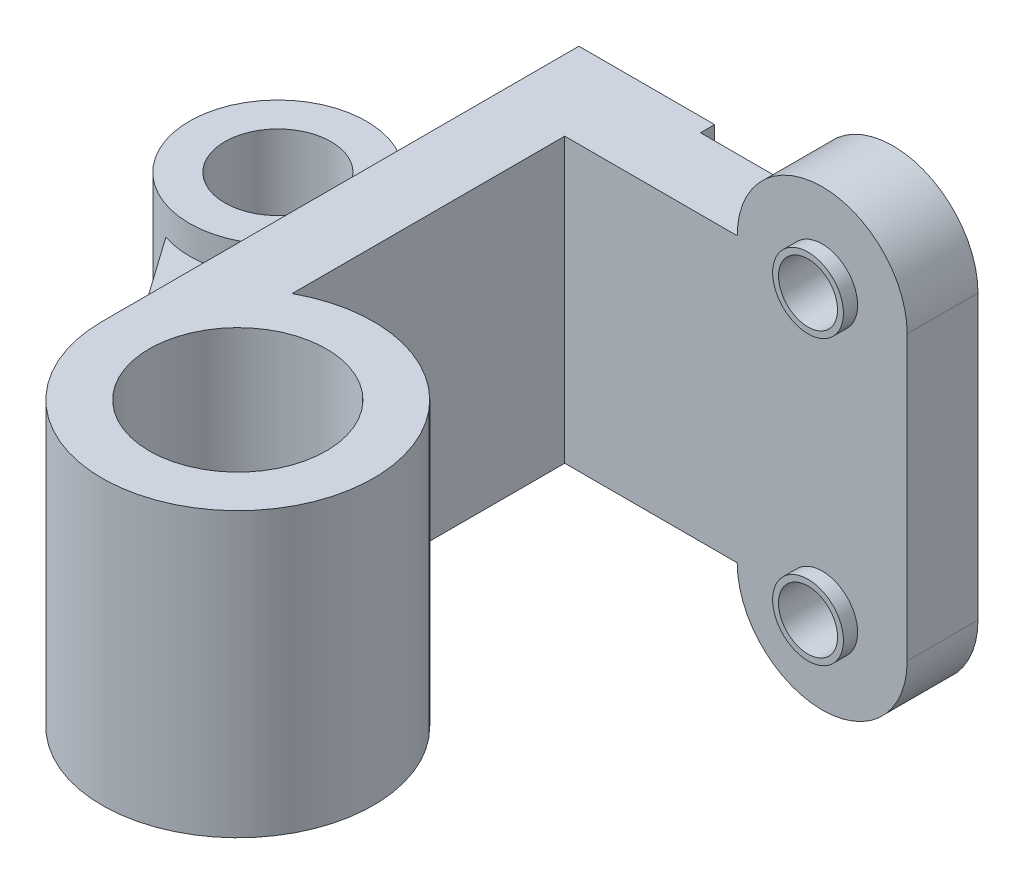
ISO-10303-21;
HEADER;
FILE_DESCRIPTION(('STEP AP214'),'2;1');
FILE_NAME('part.step','',(''),(''),'','','');
FILE_SCHEMA(('AUTOMOTIVE_DESIGN { 1 0 10303 214 1 1 1 1 }'));
ENDSEC;
DATA;
#1=APPLICATION_CONTEXT('core data for automotive mechanical design processes');
#2=APPLICATION_PROTOCOL_DEFINITION('international standard','automotive_design',2000,#1);
#3=PRODUCT_CONTEXT('',#1,'mechanical');
#4=PRODUCT('Part','Part','',(#3));
#5=PRODUCT_RELATED_PRODUCT_CATEGORY('part','',(#4));
#6=PRODUCT_DEFINITION_FORMATION('','',#4);
#7=PRODUCT_DEFINITION_CONTEXT('part definition',#1,'design');
#8=PRODUCT_DEFINITION('design','',#6,#7);
#9=PRODUCT_DEFINITION_SHAPE('','',#8);
#10=(LENGTH_UNIT() NAMED_UNIT(*) SI_UNIT(.MILLI.,.METRE.));
#11=(NAMED_UNIT(*) PLANE_ANGLE_UNIT() SI_UNIT($,.RADIAN.));
#12=(NAMED_UNIT(*) SI_UNIT($,.STERADIAN.) SOLID_ANGLE_UNIT());
#13=UNCERTAINTY_MEASURE_WITH_UNIT(LENGTH_MEASURE(1.E-05),#10,'distance_accuracy_value','');
#14=(GEOMETRIC_REPRESENTATION_CONTEXT(3) GLOBAL_UNCERTAINTY_ASSIGNED_CONTEXT((#13)) GLOBAL_UNIT_ASSIGNED_CONTEXT((#10,
#11,#12)) REPRESENTATION_CONTEXT('',''));
#15=CARTESIAN_POINT('',(0.,0.,0.));
#16=DIRECTION('',(0.,0.,1.));
#17=DIRECTION('',(1.,0.,0.));
#18=AXIS2_PLACEMENT_3D('',#15,#16,#17);
#19=CARTESIAN_POINT('',(-25.3130662470469,13.,-35.3301610889812));
#20=DIRECTION('',(0.582414315015222,0.,0.812892099645058));
#21=DIRECTION('',(0.812892099645058,0.,-0.582414315015222));
#22=AXIS2_PLACEMENT_3D('',#19,#20,#21);
#23=PLANE('',#22);
#24=DIRECTION('',(0.,-1.,0.));
#25=VECTOR('',#24,1.);
#26=CARTESIAN_POINT('',(-118.590283261648,25.,31.5003401273626));
#27=LINE('',#26,#25);
#28=CARTESIAN_POINT('',(-118.590283261648,13.,31.5003401273626));
#29=VERTEX_POINT('',#28);
#30=CARTESIAN_POINT('',(-118.590283261648,-13.,31.5003401273626));
#31=VERTEX_POINT('',#30);
#32=EDGE_CURVE('E61',#29,#31,#27,.T.);
#33=ORIENTED_EDGE('',*,*,#32,.F.);
#34=DIRECTION('',(-0.812892099645058,0.,0.582414315015222));
#35=VECTOR('',#34,1.);
#36=CARTESIAN_POINT('',(-25.3130662470469,13.,-35.3301610889812));
#37=LINE('',#36,#35);
#38=CARTESIAN_POINT('',(-66.25,13.,-6.));
#39=VERTEX_POINT('',#38);
#40=EDGE_CURVE('E170',#39,#29,#37,.T.);
#41=ORIENTED_EDGE('',*,*,#40,.F.);
#42=DIRECTION('',(0.,-1.,0.));
#43=VECTOR('',#42,1.);
#44=CARTESIAN_POINT('',(-66.25,13.,-6.));
#45=LINE('',#44,#43);
#46=CARTESIAN_POINT('',(-66.25,-13.,-6.));
#47=VERTEX_POINT('',#46);
#48=EDGE_CURVE('E175',#39,#47,#45,.T.);
#49=ORIENTED_EDGE('',*,*,#48,.T.);
#50=DIRECTION('',(-0.812892099645058,0.,0.582414315015222));
#51=VECTOR('',#50,1.);
#52=CARTESIAN_POINT('',(-25.3130662470469,-13.,-35.3301610889812));
#53=LINE('',#52,#51);
#54=EDGE_CURVE('E155',#47,#31,#53,.T.);
#55=ORIENTED_EDGE('',*,*,#54,.T.);
#56=EDGE_LOOP('',(#33,#41,#49,#55));
#57=FACE_BOUND('',#56,.T.);
#58=ADVANCED_FACE('F41',(#57),#23,.F.);
#59=CARTESIAN_POINT('',(-136.555750036393,13.,96.170909540454));
#60=DIRECTION('',(-0.81759186098535,0.,0.575798184132697));
#61=DIRECTION('',(0.575798184132697,0.,0.81759186098535));
#62=AXIS2_PLACEMENT_3D('',#59,#60,#61);
#63=PLANE('',#62);
#64=DIRECTION('',(-0.575798184132697,0.,-0.81759186098535));
#65=VECTOR('',#64,1.);
#66=CARTESIAN_POINT('',(-136.555750036393,13.,96.170909540454));
#67=LINE('',#66,#65);
#68=CARTESIAN_POINT('',(-66.25,13.,196.));
#69=VERTEX_POINT('',#68);
#70=CARTESIAN_POINT('',(-130.645274515728,13.,104.563358168141));
#71=VERTEX_POINT('',#70);
#72=EDGE_CURVE('E160',#69,#71,#67,.T.);
#73=ORIENTED_EDGE('',*,*,#72,.T.);
#74=DIRECTION('',(0.,-1.,0.));
#75=VECTOR('',#74,1.);
#76=CARTESIAN_POINT('',(-130.645274515728,25.,104.563358168141));
#77=LINE('',#76,#75);
#78=CARTESIAN_POINT('',(-130.645274515728,-13.,104.563358168141));
#79=VERTEX_POINT('',#78);
#80=EDGE_CURVE('E152',#71,#79,#77,.T.);
#81=ORIENTED_EDGE('',*,*,#80,.T.);
#82=DIRECTION('',(-0.575798184132697,0.,-0.81759186098535));
#83=VECTOR('',#82,1.);
#84=CARTESIAN_POINT('',(-136.555750036393,-13.,96.170909540454));
#85=LINE('',#84,#83);
#86=CARTESIAN_POINT('',(-66.25,-13.,196.));
#87=VERTEX_POINT('',#86);
#88=EDGE_CURVE('E144',#87,#79,#85,.T.);
#89=ORIENTED_EDGE('',*,*,#88,.F.);
#90=DIRECTION('',(0.,-1.,0.));
#91=VECTOR('',#90,1.);
#92=CARTESIAN_POINT('',(-66.25,13.,196.));
#93=LINE('',#92,#91);
#94=EDGE_CURVE('E176',#69,#87,#93,.T.);
#95=ORIENTED_EDGE('',*,*,#94,.F.);
#96=EDGE_LOOP('',(#73,#81,#89,#95));
#97=FACE_BOUND('',#96,.T.);
#98=ADVANCED_FACE('F158',(#97),#63,.T.);
#99=CARTESIAN_POINT('',(-66.25,60.,30.));
#100=DIRECTION('',(1.,0.,0.));
#101=DIRECTION('',(0.,0.,-1.));
#102=AXIS2_PLACEMENT_3D('',#99,#100,#101);
#103=PLANE('',#102);
#104=DIRECTION('',(0.,0.,-1.));
#105=VECTOR('',#104,1.);
#106=CARTESIAN_POINT('',(-66.25,-13.,0.));
#107=LINE('',#106,#105);
#108=EDGE_CURVE('E146',#87,#47,#107,.T.);
#109=ORIENTED_EDGE('',*,*,#108,.T.);
#110=DIRECTION('',(0.,-1.,0.));
#111=VECTOR('',#110,1.);
#112=CARTESIAN_POINT('',(-66.25,60.,-6.));
#113=LINE('',#112,#111);
#114=CARTESIAN_POINT('',(-66.25,-60.,-6.));
#115=VERTEX_POINT('',#114);
#116=EDGE_CURVE('E214',#47,#115,#113,.T.);
#117=ORIENTED_EDGE('',*,*,#116,.T.);
#118=DIRECTION('',(0.,0.,-1.));
#119=VECTOR('',#118,1.);
#120=CARTESIAN_POINT('',(-66.25,-60.,30.));
#121=LINE('',#120,#119);
#122=CARTESIAN_POINT('',(-66.25,-60.,196.));
#123=VERTEX_POINT('',#122);
#124=EDGE_CURVE('E285',#123,#115,#121,.T.);
#125=ORIENTED_EDGE('',*,*,#124,.F.);
#126=DIRECTION('',(0.,-1.,0.));
#127=VECTOR('',#126,1.);
#128=CARTESIAN_POINT('',(-66.25,0.,196.));
#129=LINE('',#128,#127);
#130=EDGE_CURVE('E199',#87,#123,#129,.T.);
#131=ORIENTED_EDGE('',*,*,#130,.F.);
#132=EDGE_LOOP('',(#109,#117,#125,#131));
#133=FACE_BOUND('',#132,.T.);
#134=ADVANCED_FACE('F357',(#133),#103,.F.);
#135=CARTESIAN_POINT('',(-36.25,0.,196.));
#136=DIRECTION('',(1.,0.,0.));
#137=DIRECTION('',(0.,1.,0.));
#138=AXIS2_PLACEMENT_3D('',#135,#136,#137);
#139=PLANE('',#138);
#140=DIRECTION('',(0.,0.,-1.));
#141=VECTOR('',#140,1.);
#142=CARTESIAN_POINT('',(-36.25,60.,196.));
#143=LINE('',#142,#141);
#144=CARTESIAN_POINT('',(-36.25,60.,145.50247530819));
#145=VERTEX_POINT('',#144);
#146=CARTESIAN_POINT('',(-36.25,60.,30.));
#147=VERTEX_POINT('',#146);
#148=EDGE_CURVE('E201',#145,#147,#143,.T.);
#149=ORIENTED_EDGE('',*,*,#148,.F.);
#150=DIRECTION('',(0.,-1.,0.));
#151=VECTOR('',#150,1.);
#152=CARTESIAN_POINT('',(-36.25,60.,145.50247530819));
#153=LINE('',#152,#151);
#154=CARTESIAN_POINT('',(-36.25,-60.,145.50247530819));
#155=VERTEX_POINT('',#154);
#156=EDGE_CURVE('E190',#145,#155,#153,.T.);
#157=ORIENTED_EDGE('',*,*,#156,.T.);
#158=DIRECTION('',(0.,0.,-1.));
#159=VECTOR('',#158,1.);
#160=CARTESIAN_POINT('',(-36.25,-60.,196.));
#161=LINE('',#160,#159);
#162=CARTESIAN_POINT('',(-36.25,-60.,30.));
#163=VERTEX_POINT('',#162);
#164=EDGE_CURVE('E196',#155,#163,#161,.T.);
#165=ORIENTED_EDGE('',*,*,#164,.T.);
#166=DIRECTION('',(0.,-1.,0.));
#167=VECTOR('',#166,1.);
#168=CARTESIAN_POINT('',(-36.25,0.,30.));
#169=LINE('',#168,#167);
#170=EDGE_CURVE('E191',#147,#163,#169,.T.);
#171=ORIENTED_EDGE('',*,*,#170,.F.);
#172=EDGE_LOOP('',(#149,#157,#165,#171));
#173=FACE_BOUND('',#172,.T.);
#174=ADVANCED_FACE('F321',(#173),#139,.T.);
#175=CARTESIAN_POINT('',(72.8125,60.,0.));
#176=DIRECTION('',(0.,0.,1.));
#177=DIRECTION('',(1.,0.,0.));
#178=AXIS2_PLACEMENT_3D('',#175,#176,#177);
#179=PLANE('',#178);
#180=CARTESIAN_POINT('',(72.8125,-60.,0.));
#181=DIRECTION('',(0.,0.,1.));
#182=DIRECTION('',(1.,0.,0.));
#183=AXIS2_PLACEMENT_3D('',#180,#181,#182);
#184=CIRCLE('',#183,12.5);
#185=CARTESIAN_POINT('',(85.3125,-60.,0.));
#186=VERTEX_POINT('',#185);
#187=EDGE_CURVE('E241',#186,#186,#184,.T.);
#188=ORIENTED_EDGE('',*,*,#187,.T.);
#189=EDGE_LOOP('',(#188));
#190=FACE_BOUND('',#189,.T.);
#191=CARTESIAN_POINT('',(72.8125,60.,0.));
#192=DIRECTION('',(0.,0.,1.));
#193=DIRECTION('',(1.,0.,0.));
#194=AXIS2_PLACEMENT_3D('',#191,#192,#193);
#195=CIRCLE('',#194,12.5);
#196=CARTESIAN_POINT('',(85.3125,60.,0.));
#197=VERTEX_POINT('',#196);
#198=EDGE_CURVE('E246',#197,#197,#195,.T.);
#199=ORIENTED_EDGE('',*,*,#198,.T.);
#200=EDGE_LOOP('',(#199));
#201=FACE_BOUND('',#200,.T.);
#202=DIRECTION('',(0.,-1.,0.));
#203=VECTOR('',#202,1.);
#204=CARTESIAN_POINT('',(-8.75,60.,0.));
#205=LINE('',#204,#203);
#206=CARTESIAN_POINT('',(-8.75000000000001,60.,0.));
#207=VERTEX_POINT('',#206);
#208=CARTESIAN_POINT('',(-8.75000000000001,-60.,0.));
#209=VERTEX_POINT('',#208);
#210=EDGE_CURVE('E202',#207,#209,#205,.T.);
#211=ORIENTED_EDGE('',*,*,#210,.F.);
#212=DIRECTION('',(-1.,0.,0.));
#213=VECTOR('',#212,1.);
#214=CARTESIAN_POINT('',(36.8125,60.,0.));
#215=LINE('',#214,#213);
#216=CARTESIAN_POINT('',(36.8125,60.,0.));
#217=VERTEX_POINT('',#216);
#218=EDGE_CURVE('E268',#217,#207,#215,.T.);
#219=ORIENTED_EDGE('',*,*,#218,.F.);
#220=CARTESIAN_POINT('',(72.8125,60.,0.));
#221=DIRECTION('',(0.,0.,1.));
#222=DIRECTION('',(1.,0.,0.));
#223=AXIS2_PLACEMENT_3D('',#220,#221,#222);
#224=CIRCLE('',#223,36.);
#225=CARTESIAN_POINT('',(108.8125,60.,0.));
#226=VERTEX_POINT('',#225);
#227=EDGE_CURVE('E248',#226,#217,#224,.T.);
#228=ORIENTED_EDGE('',*,*,#227,.F.);
#229=DIRECTION('',(0.,1.,0.));
#230=VECTOR('',#229,1.);
#231=CARTESIAN_POINT('',(108.8125,60.,0.));
#232=LINE('',#231,#230);
#233=CARTESIAN_POINT('',(108.8125,-60.,0.));
#234=VERTEX_POINT('',#233);
#235=EDGE_CURVE('E251',#234,#226,#232,.T.);
#236=ORIENTED_EDGE('',*,*,#235,.F.);
#237=CARTESIAN_POINT('',(72.8125,-60.,0.));
#238=DIRECTION('',(0.,0.,1.));
#239=DIRECTION('',(1.,0.,0.));
#240=AXIS2_PLACEMENT_3D('',#237,#238,#239);
#241=CIRCLE('',#240,36.);
#242=CARTESIAN_POINT('',(36.8125,-60.,0.));
#243=VERTEX_POINT('',#242);
#244=EDGE_CURVE('E272',#243,#234,#241,.T.);
#245=ORIENTED_EDGE('',*,*,#244,.F.);
#246=DIRECTION('',(1.,0.,0.));
#247=VECTOR('',#246,1.);
#248=CARTESIAN_POINT('',(-66.25,-60.,0.));
#249=LINE('',#248,#247);
#250=EDGE_CURVE('E269',#209,#243,#249,.T.);
#251=ORIENTED_EDGE('',*,*,#250,.F.);
#252=EDGE_LOOP('',(#211,#219,#228,#236,#245,#251));
#253=FACE_BOUND('',#252,.T.);
#254=ADVANCED_FACE('F296',(#190,#201,#253),#179,.F.);
#255=CARTESIAN_POINT('',(72.8125,60.,30.));
#256=DIRECTION('',(0.,0.,1.));
#257=DIRECTION('',(1.,0.,0.));
#258=AXIS2_PLACEMENT_3D('',#255,#256,#257);
#259=PLANE('',#258);
#260=ORIENTED_EDGE('',*,*,#170,.T.);
#261=DIRECTION('',(1.,0.,0.));
#262=VECTOR('',#261,1.);
#263=CARTESIAN_POINT('',(-66.25,-60.,30.));
#264=LINE('',#263,#262);
#265=CARTESIAN_POINT('',(36.8125,-60.,30.));
#266=VERTEX_POINT('',#265);
#267=EDGE_CURVE('E260',#163,#266,#264,.T.);
#268=ORIENTED_EDGE('',*,*,#267,.T.);
#269=CARTESIAN_POINT('',(72.8125,-60.,30.));
#270=DIRECTION('',(0.,0.,1.));
#271=DIRECTION('',(1.,0.,0.));
#272=AXIS2_PLACEMENT_3D('',#269,#270,#271);
#273=CIRCLE('',#272,36.);
#274=CARTESIAN_POINT('',(108.8125,-60.,30.));
#275=VERTEX_POINT('',#274);
#276=EDGE_CURVE('E256',#266,#275,#273,.T.);
#277=ORIENTED_EDGE('',*,*,#276,.T.);
#278=DIRECTION('',(0.,1.,0.));
#279=VECTOR('',#278,1.);
#280=CARTESIAN_POINT('',(108.8125,60.,30.));
#281=LINE('',#280,#279);
#282=CARTESIAN_POINT('',(108.8125,60.,30.));
#283=VERTEX_POINT('',#282);
#284=EDGE_CURVE('E263',#275,#283,#281,.T.);
#285=ORIENTED_EDGE('',*,*,#284,.T.);
#286=CARTESIAN_POINT('',(72.8125,60.,30.));
#287=DIRECTION('',(0.,0.,1.));
#288=DIRECTION('',(1.,0.,0.));
#289=AXIS2_PLACEMENT_3D('',#286,#287,#288);
#290=CIRCLE('',#289,36.);
#291=CARTESIAN_POINT('',(36.8125,60.,30.));
#292=VERTEX_POINT('',#291);
#293=EDGE_CURVE('E249',#283,#292,#290,.T.);
#294=ORIENTED_EDGE('',*,*,#293,.T.);
#295=DIRECTION('',(-1.,0.,0.));
#296=VECTOR('',#295,1.);
#297=CARTESIAN_POINT('',(36.8125,60.,30.));
#298=LINE('',#297,#296);
#299=EDGE_CURVE('E254',#292,#147,#298,.T.);
#300=ORIENTED_EDGE('',*,*,#299,.T.);
#301=EDGE_LOOP('',(#260,#268,#277,#285,#294,#300));
#302=FACE_BOUND('',#301,.T.);
#303=CARTESIAN_POINT('',(72.8125,-60.,30.));
#304=DIRECTION('',(0.,0.,1.));
#305=DIRECTION('',(1.,0.,0.));
#306=AXIS2_PLACEMENT_3D('',#303,#304,#305);
#307=CIRCLE('',#306,15.);
#308=CARTESIAN_POINT('',(87.8125,-60.,30.));
#309=VERTEX_POINT('',#308);
#310=EDGE_CURVE('E230',#309,#309,#307,.T.);
#311=ORIENTED_EDGE('',*,*,#310,.F.);
#312=EDGE_LOOP('',(#311));
#313=FACE_BOUND('',#312,.T.);
#314=CARTESIAN_POINT('',(72.8125,60.,30.));
#315=DIRECTION('',(0.,0.,1.));
#316=DIRECTION('',(1.,0.,0.));
#317=AXIS2_PLACEMENT_3D('',#314,#315,#316);
#318=CIRCLE('',#317,15.);
#319=CARTESIAN_POINT('',(87.8125,60.,30.));
#320=VERTEX_POINT('',#319);
#321=EDGE_CURVE('E232',#320,#320,#318,.T.);
#322=ORIENTED_EDGE('',*,*,#321,.F.);
#323=EDGE_LOOP('',(#322));
#324=FACE_BOUND('',#323,.T.);
#325=ADVANCED_FACE('F325',(#302,#313,#324),#259,.T.);
#326=CARTESIAN_POINT('',(72.8125,60.,30.));
#327=DIRECTION('',(0.,0.,-1.));
#328=DIRECTION('',(-1.,0.,0.));
#329=AXIS2_PLACEMENT_3D('',#326,#327,#328);
#330=CYLINDRICAL_SURFACE('',#329,36.);
#331=ORIENTED_EDGE('',*,*,#227,.T.);
#332=DIRECTION('',(0.,0.,-1.));
#333=VECTOR('',#332,1.);
#334=CARTESIAN_POINT('',(36.8125,60.,30.));
#335=LINE('',#334,#333);
#336=EDGE_CURVE('E47',#292,#217,#335,.T.);
#337=ORIENTED_EDGE('',*,*,#336,.F.);
#338=ORIENTED_EDGE('',*,*,#293,.F.);
#339=DIRECTION('',(0.,0.,-1.));
#340=VECTOR('',#339,1.);
#341=CARTESIAN_POINT('',(108.8125,60.,30.));
#342=LINE('',#341,#340);
#343=EDGE_CURVE('E261',#283,#226,#342,.T.);
#344=ORIENTED_EDGE('',*,*,#343,.T.);
#345=EDGE_LOOP('',(#331,#337,#338,#344));
#346=FACE_BOUND('',#345,.T.);
#347=ADVANCED_FACE('F43',(#346),#330,.T.);
#348=CARTESIAN_POINT('',(36.8125,60.,30.));
#349=DIRECTION('',(0.,-1.,0.));
#350=DIRECTION('',(0.,0.,-1.));
#351=AXIS2_PLACEMENT_3D('',#348,#349,#350);
#352=PLANE('',#351);
#353=DIRECTION('',(0.,0.,-1.));
#354=VECTOR('',#353,1.);
#355=CARTESIAN_POINT('',(-66.25,60.,30.));
#356=LINE('',#355,#354);
#357=CARTESIAN_POINT('',(-66.25,60.,196.));
#358=VERTEX_POINT('',#357);
#359=CARTESIAN_POINT('',(-66.25,60.,-6.));
#360=VERTEX_POINT('',#359);
#361=EDGE_CURVE('E282',#358,#360,#356,.T.);
#362=ORIENTED_EDGE('',*,*,#361,.F.);
#363=CARTESIAN_POINT('',(-8.75,60.,196.));
#364=DIRECTION('',(0.,1.,0.));
#365=DIRECTION('',(0.,0.,1.));
#366=AXIS2_PLACEMENT_3D('',#363,#364,#365);
#367=CIRCLE('',#366,57.5);
#368=EDGE_CURVE('E182',#358,#145,#367,.T.);
#369=ORIENTED_EDGE('',*,*,#368,.T.);
#370=ORIENTED_EDGE('',*,*,#148,.T.);
#371=ORIENTED_EDGE('',*,*,#299,.F.);
#372=ORIENTED_EDGE('',*,*,#336,.T.);
#373=ORIENTED_EDGE('',*,*,#218,.T.);
#374=DIRECTION('',(0.,0.,1.));
#375=VECTOR('',#374,1.);
#376=CARTESIAN_POINT('',(-8.75,60.,-6.));
#377=LINE('',#376,#375);
#378=CARTESIAN_POINT('',(-8.75,60.,-6.));
#379=VERTEX_POINT('',#378);
#380=EDGE_CURVE('E217',#379,#207,#377,.T.);
#381=ORIENTED_EDGE('',*,*,#380,.F.);
#382=DIRECTION('',(1.,0.,0.));
#383=VECTOR('',#382,1.);
#384=CARTESIAN_POINT('',(-66.25,60.,-6.));
#385=LINE('',#384,#383);
#386=EDGE_CURVE('E212',#360,#379,#385,.T.);
#387=ORIENTED_EDGE('',*,*,#386,.F.);
#388=EDGE_LOOP('',(#362,#369,#370,#371,#372,#373,#381,#387));
#389=FACE_BOUND('',#388,.T.);
#390=CARTESIAN_POINT('',(-8.75,60.,196.));
#391=DIRECTION('',(0.,1.,0.));
#392=DIRECTION('',(0.,0.,1.));
#393=AXIS2_PLACEMENT_3D('',#390,#391,#392);
#394=CIRCLE('',#393,37.5);
#395=CARTESIAN_POINT('',(-8.75,60.,233.5));
#396=VERTEX_POINT('',#395);
#397=EDGE_CURVE('E179',#396,#396,#394,.T.);
#398=ORIENTED_EDGE('',*,*,#397,.F.);
#399=EDGE_LOOP('',(#398));
#400=FACE_BOUND('',#399,.T.);
#401=ADVANCED_FACE('F289',(#389,#400),#352,.F.);
#402=EDGE_CURVE('E211',#360,#39,#113,.T.);
#403=ORIENTED_EDGE('',*,*,#402,.T.);
#404=DIRECTION('',(0.,0.,-1.));
#405=VECTOR('',#404,1.);
#406=CARTESIAN_POINT('',(-66.25,13.,0.));
#407=LINE('',#406,#405);
#408=EDGE_CURVE('E167',#69,#39,#407,.T.);
#409=ORIENTED_EDGE('',*,*,#408,.F.);
#410=EDGE_CURVE('E193',#358,#69,#129,.T.);
#411=ORIENTED_EDGE('',*,*,#410,.F.);
#412=ORIENTED_EDGE('',*,*,#361,.T.);
#413=EDGE_LOOP('',(#403,#409,#411,#412));
#414=FACE_BOUND('',#413,.T.);
#415=ADVANCED_FACE('F313',(#414),#103,.F.);
#416=CARTESIAN_POINT('',(-66.25,-60.,30.));
#417=DIRECTION('',(0.,1.,0.));
#418=DIRECTION('',(0.,0.,1.));
#419=AXIS2_PLACEMENT_3D('',#416,#417,#418);
#420=PLANE('',#419);
#421=ORIENTED_EDGE('',*,*,#164,.F.);
#422=CARTESIAN_POINT('',(-8.75,-60.,196.));
#423=DIRECTION('',(0.,1.,0.));
#424=DIRECTION('',(0.,0.,1.));
#425=AXIS2_PLACEMENT_3D('',#422,#423,#424);
#426=CIRCLE('',#425,57.5);
#427=EDGE_CURVE('E183',#123,#155,#426,.T.);
#428=ORIENTED_EDGE('',*,*,#427,.F.);
#429=ORIENTED_EDGE('',*,*,#124,.T.);
#430=DIRECTION('',(1.,0.,0.));
#431=VECTOR('',#430,1.);
#432=CARTESIAN_POINT('',(-66.25,-60.,-6.));
#433=LINE('',#432,#431);
#434=CARTESIAN_POINT('',(-8.75000000000001,-60.,-6.));
#435=VERTEX_POINT('',#434);
#436=EDGE_CURVE('E207',#115,#435,#433,.T.);
#437=ORIENTED_EDGE('',*,*,#436,.T.);
#438=DIRECTION('',(0.,0.,1.));
#439=VECTOR('',#438,1.);
#440=CARTESIAN_POINT('',(-8.75000000000001,-60.,-6.));
#441=LINE('',#440,#439);
#442=EDGE_CURVE('E220',#435,#209,#441,.T.);
#443=ORIENTED_EDGE('',*,*,#442,.T.);
#444=ORIENTED_EDGE('',*,*,#250,.T.);
#445=DIRECTION('',(0.,0.,-1.));
#446=VECTOR('',#445,1.);
#447=CARTESIAN_POINT('',(36.8125,-60.,30.));
#448=LINE('',#447,#446);
#449=EDGE_CURVE('E276',#266,#243,#448,.T.);
#450=ORIENTED_EDGE('',*,*,#449,.F.);
#451=ORIENTED_EDGE('',*,*,#267,.F.);
#452=EDGE_LOOP('',(#421,#428,#429,#437,#443,#444,#450,#451));
#453=FACE_BOUND('',#452,.T.);
#454=CARTESIAN_POINT('',(-8.75,-60.,196.));
#455=DIRECTION('',(0.,1.,0.));
#456=DIRECTION('',(0.,0.,1.));
#457=AXIS2_PLACEMENT_3D('',#454,#455,#456);
#458=CIRCLE('',#457,37.5);
#459=CARTESIAN_POINT('',(-8.75,-60.,233.5));
#460=VERTEX_POINT('',#459);
#461=EDGE_CURVE('E177',#460,#460,#458,.T.);
#462=ORIENTED_EDGE('',*,*,#461,.T.);
#463=EDGE_LOOP('',(#462));
#464=FACE_BOUND('',#463,.T.);
#465=ADVANCED_FACE('F329',(#453,#464),#420,.F.);
#466=CARTESIAN_POINT('',(72.8125,-60.,30.));
#467=DIRECTION('',(0.,0.,-1.));
#468=DIRECTION('',(-1.,0.,0.));
#469=AXIS2_PLACEMENT_3D('',#466,#467,#468);
#470=CYLINDRICAL_SURFACE('',#469,36.);
#471=ORIENTED_EDGE('',*,*,#244,.T.);
#472=DIRECTION('',(0.,0.,-1.));
#473=VECTOR('',#472,1.);
#474=CARTESIAN_POINT('',(108.8125,-60.,30.));
#475=LINE('',#474,#473);
#476=EDGE_CURVE('E277',#275,#234,#475,.T.);
#477=ORIENTED_EDGE('',*,*,#476,.F.);
#478=ORIENTED_EDGE('',*,*,#276,.F.);
#479=ORIENTED_EDGE('',*,*,#449,.T.);
#480=EDGE_LOOP('',(#471,#477,#478,#479));
#481=FACE_BOUND('',#480,.T.);
#482=ADVANCED_FACE('F332',(#481),#470,.T.);
#483=CARTESIAN_POINT('',(108.8125,60.,30.));
#484=DIRECTION('',(-1.,0.,0.));
#485=DIRECTION('',(0.,0.,1.));
#486=AXIS2_PLACEMENT_3D('',#483,#484,#485);
#487=PLANE('',#486);
#488=ORIENTED_EDGE('',*,*,#235,.T.);
#489=ORIENTED_EDGE('',*,*,#343,.F.);
#490=ORIENTED_EDGE('',*,*,#284,.F.);
#491=ORIENTED_EDGE('',*,*,#476,.T.);
#492=EDGE_LOOP('',(#488,#489,#490,#491));
#493=FACE_BOUND('',#492,.T.);
#494=ADVANCED_FACE('F340',(#493),#487,.F.);
#495=CARTESIAN_POINT('',(72.8125,60.,30.));
#496=DIRECTION('',(0.,0.,-1.));
#497=DIRECTION('',(-1.,0.,0.));
#498=AXIS2_PLACEMENT_3D('',#495,#496,#497);
#499=CYLINDRICAL_SURFACE('',#498,12.5);
#500=ORIENTED_EDGE('',*,*,#198,.F.);
#501=EDGE_LOOP('',(#500));
#502=FACE_BOUND('',#501,.T.);
#503=CARTESIAN_POINT('',(72.8125,60.,36.));
#504=DIRECTION('',(0.,0.,-1.));
#505=DIRECTION('',(-1.,0.,0.));
#506=AXIS2_PLACEMENT_3D('',#503,#504,#505);
#507=CIRCLE('',#506,12.5);
#508=CARTESIAN_POINT('',(60.3125,60.,36.));
#509=VERTEX_POINT('',#508);
#510=EDGE_CURVE('E228',#509,#509,#507,.T.);
#511=ORIENTED_EDGE('',*,*,#510,.F.);
#512=EDGE_LOOP('',(#511));
#513=FACE_BOUND('',#512,.T.);
#514=ADVANCED_FACE('F339',(#502,#513),#499,.F.);
#515=CARTESIAN_POINT('',(72.8125,-60.,30.));
#516=DIRECTION('',(0.,0.,-1.));
#517=DIRECTION('',(-1.,0.,0.));
#518=AXIS2_PLACEMENT_3D('',#515,#516,#517);
#519=CYLINDRICAL_SURFACE('',#518,12.5);
#520=ORIENTED_EDGE('',*,*,#187,.F.);
#521=EDGE_LOOP('',(#520));
#522=FACE_BOUND('',#521,.T.);
#523=CARTESIAN_POINT('',(72.8125,-60.,36.));
#524=DIRECTION('',(0.,0.,-1.));
#525=DIRECTION('',(-1.,0.,0.));
#526=AXIS2_PLACEMENT_3D('',#523,#524,#525);
#527=CIRCLE('',#526,12.5);
#528=CARTESIAN_POINT('',(60.3125,-60.,36.));
#529=VERTEX_POINT('',#528);
#530=EDGE_CURVE('E221',#529,#529,#527,.T.);
#531=ORIENTED_EDGE('',*,*,#530,.F.);
#532=EDGE_LOOP('',(#531));
#533=FACE_BOUND('',#532,.T.);
#534=ADVANCED_FACE('F348',(#522,#533),#519,.F.);
#535=CARTESIAN_POINT('',(72.8125,60.,36.));
#536=DIRECTION('',(0.,0.,-1.));
#537=DIRECTION('',(-1.,0.,0.));
#538=AXIS2_PLACEMENT_3D('',#535,#536,#537);
#539=CYLINDRICAL_SURFACE('',#538,15.);
#540=CARTESIAN_POINT('',(72.8125,60.,36.));
#541=DIRECTION('',(0.,0.,1.));
#542=DIRECTION('',(1.,0.,0.));
#543=AXIS2_PLACEMENT_3D('',#540,#541,#542);
#544=CIRCLE('',#543,15.);
#545=CARTESIAN_POINT('',(87.8125,60.,36.));
#546=VERTEX_POINT('',#545);
#547=EDGE_CURVE('E238',#546,#546,#544,.T.);
#548=ORIENTED_EDGE('',*,*,#547,.F.);
#549=EDGE_LOOP('',(#548));
#550=FACE_BOUND('',#549,.T.);
#551=ORIENTED_EDGE('',*,*,#321,.T.);
#552=EDGE_LOOP('',(#551));
#553=FACE_BOUND('',#552,.T.);
#554=ADVANCED_FACE('F381',(#550,#553),#539,.T.);
#555=CARTESIAN_POINT('',(72.8125,60.,36.));
#556=DIRECTION('',(0.,0.,1.));
#557=DIRECTION('',(1.,0.,0.));
#558=AXIS2_PLACEMENT_3D('',#555,#556,#557);
#559=PLANE('',#558);
#560=ORIENTED_EDGE('',*,*,#510,.T.);
#561=EDGE_LOOP('',(#560));
#562=FACE_BOUND('',#561,.T.);
#563=ORIENTED_EDGE('',*,*,#547,.T.);
#564=EDGE_LOOP('',(#563));
#565=FACE_BOUND('',#564,.T.);
#566=ADVANCED_FACE('F379',(#562,#565),#559,.T.);
#567=CARTESIAN_POINT('',(72.8125,-60.,36.));
#568=DIRECTION('',(0.,0.,-1.));
#569=DIRECTION('',(-1.,0.,0.));
#570=AXIS2_PLACEMENT_3D('',#567,#568,#569);
#571=CYLINDRICAL_SURFACE('',#570,15.);
#572=CARTESIAN_POINT('',(72.8125,-60.,36.));
#573=DIRECTION('',(0.,0.,1.));
#574=DIRECTION('',(1.,0.,0.));
#575=AXIS2_PLACEMENT_3D('',#572,#573,#574);
#576=CIRCLE('',#575,15.);
#577=CARTESIAN_POINT('',(87.8125,-60.,36.));
#578=VERTEX_POINT('',#577);
#579=EDGE_CURVE('E235',#578,#578,#576,.T.);
#580=ORIENTED_EDGE('',*,*,#579,.F.);
#581=EDGE_LOOP('',(#580));
#582=FACE_BOUND('',#581,.T.);
#583=ORIENTED_EDGE('',*,*,#310,.T.);
#584=EDGE_LOOP('',(#583));
#585=FACE_BOUND('',#584,.T.);
#586=ADVANCED_FACE('F376',(#582,#585),#571,.T.);
#587=CARTESIAN_POINT('',(72.8125,-60.,36.));
#588=DIRECTION('',(0.,0.,1.));
#589=DIRECTION('',(1.,0.,0.));
#590=AXIS2_PLACEMENT_3D('',#587,#588,#589);
#591=PLANE('',#590);
#592=ORIENTED_EDGE('',*,*,#530,.T.);
#593=EDGE_LOOP('',(#592));
#594=FACE_BOUND('',#593,.T.);
#595=ORIENTED_EDGE('',*,*,#579,.T.);
#596=EDGE_LOOP('',(#595));
#597=FACE_BOUND('',#596,.T.);
#598=ADVANCED_FACE('F373',(#594,#597),#591,.T.);
#599=CARTESIAN_POINT('',(-8.75,60.,-6.));
#600=DIRECTION('',(-1.,0.,0.));
#601=DIRECTION('',(0.,-1.,0.));
#602=AXIS2_PLACEMENT_3D('',#599,#600,#601);
#603=PLANE('',#602);
#604=ORIENTED_EDGE('',*,*,#210,.T.);
#605=ORIENTED_EDGE('',*,*,#442,.F.);
#606=DIRECTION('',(0.,-1.,0.));
#607=VECTOR('',#606,1.);
#608=CARTESIAN_POINT('',(-8.75,60.,-6.));
#609=LINE('',#608,#607);
#610=EDGE_CURVE('E209',#379,#435,#609,.T.);
#611=ORIENTED_EDGE('',*,*,#610,.F.);
#612=ORIENTED_EDGE('',*,*,#380,.T.);
#613=EDGE_LOOP('',(#604,#605,#611,#612));
#614=FACE_BOUND('',#613,.T.);
#615=ADVANCED_FACE('F305',(#614),#603,.F.);
#616=CARTESIAN_POINT('',(0.,0.,-6.));
#617=DIRECTION('',(0.,0.,-1.));
#618=DIRECTION('',(-1.,0.,0.));
#619=AXIS2_PLACEMENT_3D('',#616,#617,#618);
#620=PLANE('',#619);
#621=ORIENTED_EDGE('',*,*,#436,.F.);
#622=ORIENTED_EDGE('',*,*,#116,.F.);
#623=ORIENTED_EDGE('',*,*,#48,.F.);
#624=ORIENTED_EDGE('',*,*,#402,.F.);
#625=ORIENTED_EDGE('',*,*,#386,.T.);
#626=ORIENTED_EDGE('',*,*,#610,.T.);
#627=EDGE_LOOP('',(#621,#622,#623,#624,#625,#626));
#628=FACE_BOUND('',#627,.T.);
#629=ADVANCED_FACE('F309',(#628),#620,.T.);
#630=CARTESIAN_POINT('',(-8.75,60.,196.));
#631=DIRECTION('',(0.,-1.,0.));
#632=DIRECTION('',(0.,0.,-1.));
#633=AXIS2_PLACEMENT_3D('',#630,#631,#632);
#634=CYLINDRICAL_SURFACE('',#633,37.5);
#635=ORIENTED_EDGE('',*,*,#397,.T.);
#636=EDGE_LOOP('',(#635));
#637=FACE_BOUND('',#636,.T.);
#638=ORIENTED_EDGE('',*,*,#461,.F.);
#639=EDGE_LOOP('',(#638));
#640=FACE_BOUND('',#639,.T.);
#641=ADVANCED_FACE('F361',(#637,#640),#634,.F.);
#642=CARTESIAN_POINT('',(-8.75,60.,196.));
#643=DIRECTION('',(0.,-1.,0.));
#644=DIRECTION('',(0.,0.,-1.));
#645=AXIS2_PLACEMENT_3D('',#642,#643,#644);
#646=CYLINDRICAL_SURFACE('',#645,57.5);
#647=ORIENTED_EDGE('',*,*,#156,.F.);
#648=ORIENTED_EDGE('',*,*,#368,.F.);
#649=ORIENTED_EDGE('',*,*,#410,.T.);
#650=ORIENTED_EDGE('',*,*,#94,.T.);
#651=ORIENTED_EDGE('',*,*,#130,.T.);
#652=ORIENTED_EDGE('',*,*,#427,.T.);
#653=EDGE_LOOP('',(#647,#648,#649,#650,#651,#652));
#654=FACE_BOUND('',#653,.T.);
#655=ADVANCED_FACE('F319',(#654),#646,.T.);
#656=CARTESIAN_POINT('',(0.,13.,0.));
#657=DIRECTION('',(0.,1.,0.));
#658=DIRECTION('',(0.,0.,1.));
#659=AXIS2_PLACEMENT_3D('',#656,#657,#658);
#660=PLANE('',#659);
#661=ORIENTED_EDGE('',*,*,#40,.T.);
#662=CARTESIAN_POINT('',(-118.75,13.,69.));
#663=DIRECTION('',(0.,1.,0.));
#664=DIRECTION('',(0.,0.,1.));
#665=AXIS2_PLACEMENT_3D('',#662,#663,#664);
#666=CIRCLE('',#665,37.5);
#667=EDGE_CURVE('E57',#29,#71,#666,.F.);
#668=ORIENTED_EDGE('',*,*,#667,.T.);
#669=ORIENTED_EDGE('',*,*,#72,.F.);
#670=ORIENTED_EDGE('',*,*,#408,.T.);
#671=EDGE_LOOP('',(#661,#668,#669,#670));
#672=FACE_BOUND('',#671,.T.);
#673=ADVANCED_FACE('F365',(#672),#660,.T.);
#674=CARTESIAN_POINT('',(0.,-13.,0.));
#675=DIRECTION('',(0.,1.,0.));
#676=DIRECTION('',(0.,0.,1.));
#677=AXIS2_PLACEMENT_3D('',#674,#675,#676);
#678=PLANE('',#677);
#679=CARTESIAN_POINT('',(-118.75,-13.,69.));
#680=DIRECTION('',(0.,1.,0.));
#681=DIRECTION('',(0.,0.,1.));
#682=AXIS2_PLACEMENT_3D('',#679,#680,#681);
#683=CIRCLE('',#682,37.5);
#684=EDGE_CURVE('E11',#31,#79,#683,.F.);
#685=ORIENTED_EDGE('',*,*,#684,.F.);
#686=ORIENTED_EDGE('',*,*,#54,.F.);
#687=ORIENTED_EDGE('',*,*,#108,.F.);
#688=ORIENTED_EDGE('',*,*,#88,.T.);
#689=EDGE_LOOP('',(#685,#686,#687,#688));
#690=FACE_BOUND('',#689,.T.);
#691=ADVANCED_FACE('F147',(#690),#678,.F.);
#692=CARTESIAN_POINT('',(-118.75,25.,69.));
#693=DIRECTION('',(0.,-1.,0.));
#694=DIRECTION('',(0.,0.,-1.));
#695=AXIS2_PLACEMENT_3D('',#692,#693,#694);
#696=CYLINDRICAL_SURFACE('',#695,22.5);
#697=CARTESIAN_POINT('',(-118.75,-25.,69.));
#698=DIRECTION('',(0.,1.,0.));
#699=DIRECTION('',(0.,0.,1.));
#700=AXIS2_PLACEMENT_3D('',#697,#698,#699);
#701=CIRCLE('',#700,22.5);
#702=CARTESIAN_POINT('',(-118.75,-25.,91.5));
#703=VERTEX_POINT('',#702);
#704=EDGE_CURVE('E652',#703,#703,#701,.T.);
#705=ORIENTED_EDGE('',*,*,#704,.F.);
#706=EDGE_LOOP('',(#705));
#707=FACE_BOUND('',#706,.T.);
#708=CARTESIAN_POINT('',(-118.75,25.,69.));
#709=DIRECTION('',(0.,1.,0.));
#710=DIRECTION('',(0.,0.,1.));
#711=AXIS2_PLACEMENT_3D('',#708,#709,#710);
#712=CIRCLE('',#711,22.5);
#713=CARTESIAN_POINT('',(-118.75,25.,91.5));
#714=VERTEX_POINT('',#713);
#715=EDGE_CURVE('E658',#714,#714,#712,.T.);
#716=ORIENTED_EDGE('',*,*,#715,.T.);
#717=EDGE_LOOP('',(#716));
#718=FACE_BOUND('',#717,.T.);
#719=ADVANCED_FACE('F592',(#707,#718),#696,.F.);
#720=CARTESIAN_POINT('',(-118.75,25.,69.));
#721=DIRECTION('',(0.,1.,0.));
#722=DIRECTION('',(0.,0.,1.));
#723=AXIS2_PLACEMENT_3D('',#720,#721,#722);
#724=PLANE('',#723);
#725=CARTESIAN_POINT('',(-118.75,25.,69.));
#726=DIRECTION('',(0.,1.,0.));
#727=DIRECTION('',(0.,0.,1.));
#728=AXIS2_PLACEMENT_3D('',#725,#726,#727);
#729=CIRCLE('',#728,37.5);
#730=CARTESIAN_POINT('',(-118.75,25.,106.5));
#731=VERTEX_POINT('',#730);
#732=EDGE_CURVE('E159',#731,#731,#729,.T.);
#733=ORIENTED_EDGE('',*,*,#732,.T.);
#734=EDGE_LOOP('',(#733));
#735=FACE_BOUND('',#734,.T.);
#736=ORIENTED_EDGE('',*,*,#715,.F.);
#737=EDGE_LOOP('',(#736));
#738=FACE_BOUND('',#737,.T.);
#739=ADVANCED_FACE('F615',(#735,#738),#724,.T.);
#740=CARTESIAN_POINT('',(-118.75,-25.,69.));
#741=DIRECTION('',(0.,1.,0.));
#742=DIRECTION('',(0.,0.,1.));
#743=AXIS2_PLACEMENT_3D('',#740,#741,#742);
#744=PLANE('',#743);
#745=CARTESIAN_POINT('',(-118.75,-25.,69.));
#746=DIRECTION('',(0.,1.,0.));
#747=DIRECTION('',(0.,0.,1.));
#748=AXIS2_PLACEMENT_3D('',#745,#746,#747);
#749=CIRCLE('',#748,37.5);
#750=CARTESIAN_POINT('',(-118.75,-25.,106.5));
#751=VERTEX_POINT('',#750);
#752=EDGE_CURVE('E655',#751,#751,#749,.T.);
#753=ORIENTED_EDGE('',*,*,#752,.F.);
#754=EDGE_LOOP('',(#753));
#755=FACE_BOUND('',#754,.T.);
#756=ORIENTED_EDGE('',*,*,#704,.T.);
#757=EDGE_LOOP('',(#756));
#758=FACE_BOUND('',#757,.T.);
#759=ADVANCED_FACE('F625',(#755,#758),#744,.F.);
#760=CARTESIAN_POINT('',(-118.75,25.,69.));
#761=DIRECTION('',(0.,-1.,0.));
#762=DIRECTION('',(0.,0.,-1.));
#763=AXIS2_PLACEMENT_3D('',#760,#761,#762);
#764=CYLINDRICAL_SURFACE('',#763,37.5);
#765=ORIENTED_EDGE('',*,*,#667,.F.);
#766=ORIENTED_EDGE('',*,*,#32,.T.);
#767=ORIENTED_EDGE('',*,*,#684,.T.);
#768=ORIENTED_EDGE('',*,*,#80,.F.);
#769=EDGE_LOOP('',(#765,#766,#767,#768));
#770=FACE_BOUND('',#769,.T.);
#771=ORIENTED_EDGE('',*,*,#732,.F.);
#772=EDGE_LOOP('',(#771));
#773=FACE_BOUND('',#772,.T.);
#774=ORIENTED_EDGE('',*,*,#752,.T.);
#775=EDGE_LOOP('',(#774));
#776=FACE_BOUND('',#775,.T.);
#777=ADVANCED_FACE('F163',(#770,#773,#776),#764,.T.);
#778=CLOSED_SHELL('',(#58,#98,#134,#174,#254,#325,#347,#401,#415,#465,#482,#494,#514,#534,#554,
#566,#586,#598,#615,#629,#641,#655,#673,#691,#719,#739,#759,#777));
#779=MANIFOLD_SOLID_BREP('B2',#778);
#780=ADVANCED_BREP_SHAPE_REPRESENTATION('',(#18,#779),#14);
#781=SHAPE_DEFINITION_REPRESENTATION(#9,#780);
ENDSEC;
END-ISO-10303-21;
